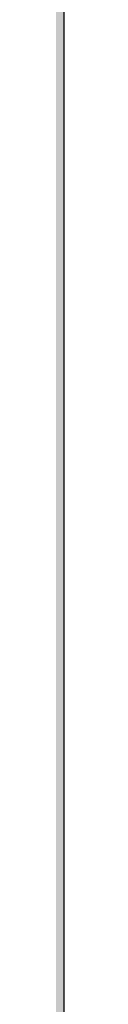
# Model space of a CAD drawing. Units: inches. Extents: x 2091 to 2899, y 967 to 2217.
# Tile 76 of 256: x 2212 to 2212, y 1105 to 1114. Entities that reach past the tile are written whole.
import ezdxf

# ---------------------------------------------------------------- set-up
doc = ezdxf.new("R2010")
doc.units = ezdxf.units.IN
doc.layers.add('A-ANNO-DIMS', color=2, linetype='Continuous', lineweight=18)
doc.layers.add('A-WALL-PATT', color=141, linetype='Continuous', lineweight=13, true_color=0xadddf7)
doc.styles.get("Standard").update_dxf_attribs({"font": 'arial.ttf'})
doc.dimstyles.new('ISO-25', dxfattribs={"dimtxt": 4, "dimasz": 4, "dimexe": 1.25, "dimexo": 0.625, "dimtad": 1, "dimdec": 0, "dimlunit": 3, "dimtxsty": 'Standard', "dimcen": 2.5, "dimadec": 0, "dimazin": 0, "dimtfac": 1, "dimtdec": 0, "dimtmove": 0, "dimatfit": 3, "dimfxl": 1, "dimarcsym": 0})

# ---------------------------------------------------------------- blocks, each defined once
blk = doc.blocks.new('*D71')
at = {"layer": 'A-ANNO-DIMS', "color": 0, "lineweight": -2, "transparency": 16777216}
for p, q in [((2212.1436, 1351.2941), (2212.1436, 969.4643)), ((2452.1436, 1351.2941), (2452.1436, 969.4643)), ((2216.1436, 970.7143), (2448.1436, 970.7143))]:
    blk.add_line(p, q, dxfattribs=at)
at = {"layer": 'A-ANNO-DIMS', "color": 0, "transparency": 16777216}
for points in [[(2216.1436, 971.381), (2216.1436, 970.0476), (2212.1436, 970.7143)], [(2448.1436, 971.381), (2448.1436, 970.0476), (2452.1436, 970.7143)]]:
    blk.add_solid(points, dxfattribs=at)
at = {"layer": 'Defpoints', "color": 0, "transparency": 16777216}
for p in [(2212.1436, 1351.9191), (2452.1436, 1351.9191), (2452.1436, 970.7143)]:
    blk.add_point(p, dxfattribs=at)
at = {"layer": 'A-ANNO-DIMS', "color": 0, "transparency": 16777216, "insert": (2332.1436, 973.3816), "char_height": 4, "attachment_point": 5}
blk.add_mtext('20\'-0"', dxfattribs=at)
blk = doc.blocks.new('*D75')
at = {"layer": 'A-ANNO-DIMS', "color": 0, "lineweight": -2, "transparency": 16777216}
for p, q in [((2212.1436, 1274.7941), (2212.1436, 969.4643)), ((2308.1436, 1274.7941), (2308.1436, 969.4643)), ((2216.1436, 970.7143), (2304.1436, 970.7143))]:
    blk.add_line(p, q, dxfattribs=at)
at = {"layer": 'A-ANNO-DIMS', "color": 0, "transparency": 16777216}
for points in [[(2216.1436, 971.381), (2216.1436, 970.0476), (2212.1436, 970.7143)], [(2304.1436, 971.381), (2304.1436, 970.0476), (2308.1436, 970.7143)]]:
    blk.add_solid(points, dxfattribs=at)
at = {"layer": 'Defpoints', "color": 0, "transparency": 16777216}
for p in [(2212.1436, 1275.4191), (2308.1436, 1275.4191), (2308.1436, 970.7143)]:
    blk.add_point(p, dxfattribs=at)
at = {"layer": 'A-ANNO-DIMS', "color": 0, "transparency": 16777216, "insert": (2260.1436, 973.3816), "char_height": 4, "attachment_point": 5}
blk.add_mtext('8\'-0"', dxfattribs=at)
blk = doc.blocks.new('*D91')
at = {"layer": 'A-ANNO-DIMS', "color": 0, "lineweight": -2, "transparency": 16777216}
for p, q in [((2211.6506, 1152.2471), (2098.3113, 1152.2471)), ((2099.5613, 1103.9191), (2099.5613, 1148.2471)), ((2211.5186, 1099.9191), (2098.3113, 1099.9191))]:
    blk.add_line(p, q, dxfattribs=at)
at = {"layer": 'A-ANNO-DIMS', "color": 0, "transparency": 16777216}
for points in [[(2098.8947, 1148.2471), (2100.228, 1148.2471), (2099.5613, 1152.2471)], [(2098.8947, 1103.9191), (2100.228, 1103.9191), (2099.5613, 1099.9191)]]:
    blk.add_solid(points, dxfattribs=at)
at = {"layer": 'Defpoints', "color": 0, "transparency": 16777216}
for p in [(2099.5613, 1152.2471), (2212.2756, 1152.2471), (2212.1436, 1099.9191)]:
    blk.add_point(p, dxfattribs=at)
at = {"layer": 'A-ANNO-DIMS', "color": 0, "transparency": 16777216, "insert": (2096.8681, 1126.0831), "char_height": 4, "attachment_point": 5, "rotation": 90}
blk.add_mtext('4\'-4 1/2"', dxfattribs=at)

msp = doc.modelspace()

# ---------------------------------------------------------------- hatches: boundary and pattern name
at = {"layer": 'A-WALL-PATT'}
h = msp.add_hatch(color=256, dxfattribs=at)
h.dxf.hatch_style = 1
h.paths.add_polyline_path([(2803.1436, 2050.9191), (2203.1436, 2050.9191), (2203.1436, 1090.9191), (2803.1436, 1090.9191)])
h.paths.add_polyline_path([(2635.7989, 1147.5405), (2674.5241, 1147.5405, 0.376086), (2678.5297, 1152.8802), (2678.5297, 1159.5565, 0.333335), (2674.5243, 1163.5618), (2674.5243, 1163.5619), (2674.5243, 1192.9344), (2635.806, 1192.9344), (2597.0876, 1192.9344), (2597.0876, 1163.5618, 0.333335), (2593.0823, 1159.5565), (2593.0823, 1152.8802, 0.376086), (2597.0879, 1147.5405)], flags=0)
h.paths.add_polyline_path([(2436.0104, 1278.2408, 0.000483), (2435.9526, 1278.215, -0.001328), (2435.9356, 1278.1117, -0.001711), (2436.1164, 1278.0408, 0.002185)], flags=0)
h.paths.add_polyline_path([(2794.1436, 1143.4191), (2794.1436, 1347.4191), (2543.3702, 1347.4191), (2543.3702, 1351.9191), (2794.1436, 1351.9191), (2794.1436, 1392.7136), (2793.9474, 1392.7136), (2793.9474, 1473.5369), (2794.1436, 1473.5369), (2794.1436, 1531.9191), (2650.1436, 1531.9191), (2650.1436, 1536.4191), (2794.1436, 1536.4191), (2794.1436, 1692.4191), (2609.3756, 1692.4191), (2609.3756, 1644.4191), (2604.8756, 1644.4191), (2604.8756, 1744.9191), (2609.3756, 1744.9191), (2609.3756, 1696.9191), (2794.1436, 1696.9191), (2794.1436, 1780.9191), (2609.6436, 1780.9191), (2493.8756, 1780.9191), (2493.8756, 1785.4191), (2609.6436, 1785.4191), (2794.1436, 1785.4191), (2794.1436, 1847.9388), (2793.9512, 1847.9388), (2793.9512, 1928.7622), (2794.1436, 1928.7622), (2794.1436, 1941.4191), (2614.1436, 1941.4191), (2614.1436, 1821.4191), (2609.6436, 1821.4191), (2609.6436, 1941.4191), (2392.1436, 1941.4191), (2392.1436, 1819.9191), (2387.6436, 1819.9191), (2387.6436, 1941.4191), (2212.1436, 1941.4191), (2212.1436, 1783.9191), (2392.1436, 1783.9191), (2392.1436, 1780.9191), (2212.1436, 1780.9191), (2212.1436, 1629.4191), (2387.6436, 1629.4191), (2387.6436, 1744.9191), (2392.1436, 1744.9191), (2392.1436, 1627.9191), (2317.1436, 1627.9191), (2317.1436, 1551.4191), (2317.1436, 1536.4191), (2459.3836, 1536.4191), (2459.3836, 1602.3965), (2463.8836, 1602.3965), (2463.8836, 1531.9191), (2456.6436, 1531.9191), (2456.6436, 1529.9191), (2452.1436, 1529.9191), (2452.1436, 1531.9191), (2312.6436, 1531.9191), (2312.6436, 1551.4191), (2306.1436, 1551.4191), (2306.1436, 1555.9191), (2308.1436, 1555.9191), (2308.1436, 1551.4191), (2312.6436, 1551.4191), (2312.6436, 1627.9191), (2212.1436, 1627.9191), (2212.1436, 1555.9191), (2270.1436, 1555.9191), (2270.1436, 1551.4191), (2212.1436, 1551.4191), (2212.1436, 1351.9191), (2272.1436, 1351.9191), (2272.1436, 1347.4191), (2212.1436, 1347.4191), (2212.1436, 1275.4191), (2308.1436, 1275.4191), (2308.1436, 1351.9191), (2452.1436, 1351.9191), (2452.1436, 1493.9191), (2456.6436, 1493.9191), (2456.6436, 1347.4191), (2312.6436, 1347.4191), (2312.6436, 1270.9191), (2212.1436, 1270.9191), (2212.1436, 1099.9191), (2281.2375, 1099.9191), (2282.871, 1110.9138), (2282.0083, 1116.9966), (2278.5577, 1121.4204), (2268.2056, 1128.0562), (2272.0876, 1128.0562), (2273.8129, 1131.927), (2279.4203, 1134.6919), (2285.0278, 1135.2449), (2287.6158, 1137.4568), (2288.0471, 1138.0098), (2289.3411, 1140.7747), (2291.0665, 1139.6687), (2292.3605, 1135.2449), (2295.3798, 1136.9038), (2296.2425, 1135.7979), (2297.1052, 1133.033), (2300.1246, 1138.0098), (2303.1439, 1138.0098), (2304.4379, 1135.7979), (2303.1439, 1133.586), (2306.5946, 1134.6919), (2307.8887, 1133.033), (2310.908, 1135.2449), (2313.9274, 1134.1389), (2315.6269, 1132.4271), (2308.32, 1117.5496), (2290.2038, 1109.8079), (2288.9098, 1103.1721), (2289.2723, 1099.9191), (2434.9182, 1099.9191), (2431.5932, 1124.7881), (2429.9302, 1169.5531), (2430.9272, 1240.5197), (2435.6589, 1238.1861), (2437.1352, 1196.5541), (2438.7982, 1143.9731), (2442.6782, 1111.9981), (2446.5582, 1099.9191), (2794.1436, 1099.9191), (2794.1436, 1138.9191), (2548.0324, 1138.9191), (2548.0324, 1143.4191), (2548.0324, 1148.8191), (2546.6685, 1148.0316), (2528.6857, 1179.1786, 0.256256), (2512.0324, 1148.8191), (2512.0324, 1143.4191), (2512.0324, 1138.9191), (2507.5324, 1138.9191), (2507.5324, 1143.4191), (2507.5324, 1148.8191, 0.256256), (2490.8792, 1179.1786), (2472.8964, 1148.0316), (2471.5324, 1148.8191), (2471.5324, 1143.4191), (2467.0324, 1143.4191), (2467.0324, 1269.9458, 0.039061), (2460.91, 1273.5801), (2467.0324, 1273.5801), (2467.0324, 1286.3254, 0.014511), (2465.2162, 1286.7619), (2467.0324, 1287.0526), (2467.0324, 1323.4191), (2471.5324, 1323.4191), (2471.5324, 1148.8191), (2489.5324, 1179.996), (2490.8964, 1179.2085), (2490.8792, 1179.1786, -0.256256), (2507.5324, 1148.8191), (2507.5324, 1143.4191), (2512.0324, 1143.4191), (2512.0324, 1148.8191, -0.256256), (2528.6857, 1179.1786), (2528.6685, 1179.2085), (2530.0324, 1179.996), (2548.0324, 1148.8191), (2548.0324, 1143.4191)], flags=16)
h.paths.add_polyline_path([(2607.7685, 1200.9451), (2607.7685, 1265.0306), (2597.0876, 1281.052), (2619.7846, 1281.052), (2627.7953, 1337.1269), (2635.7989, 1337.1269), (2643.8167, 1337.1269), (2651.8274, 1281.052), (2674.5243, 1281.052), (2663.8434, 1265.0306), (2663.8434, 1200.9451), (2635.806, 1200.9451)], flags=0)
edge = h.paths.add_edge_path(flags=0)
edge.add_ellipse((13303.8962, 1272.9987), major_axis=(-10595.313, 0), ratio=0.8423038701, start_angle=0.62823722, end_angle=0.6465541, ccw=False)
edge.add_ellipse((2711.7004, 1156.8527), major_axis=(2.2198, 0), ratio=0.842304, start_angle=111.53524, end_angle=180.62824, ccw=False)
edge.add_ellipse((13303.1563, 1272.9987), major_axis=(-10593.0263, 0), ratio=0.8423038695, start_angle=0.52827147, end_angle=0.6465541, ccw=False)
edge.add_line((2710.7646, 1175.3333), (2710.13, 1175.3333))
edge.add_ellipse((2710.13, 1176.5798), major_axis=(1.4798, 0), ratio=0.842304, start_angle=180, end_angle=270, ccw=False)
edge.add_line((2708.6501, 1176.5798), (2708.6501, 1200.7829))
edge.add_ellipse((2710.13, 1200.7829), major_axis=(1.4798, 0), ratio=0.842304, start_angle=90, end_angle=180, ccw=False)
edge.add_line((2710.13, 1202.0294), (2710.4651, 1202.0294))
edge.add_ellipse((13303.1563, 1272.9987), major_axis=(-10593.0263, 0), ratio=0.8423038695, start_angle=-0.09022909, end_angle=0.38386678, ccw=False)
edge.add_ellipse((2710.13, 1290.927), major_axis=(-1.4798, 0), ratio=0.842304, start_angle=0, end_angle=90, ccw=False)
edge.add_line((2708.6501, 1290.927), (2708.6501, 1315.1302))
edge.add_ellipse((2710.13, 1315.1302), major_axis=(-1.4798, 0), ratio=0.842304, start_angle=-90, end_angle=0, ccw=False)
edge.add_line((2710.13, 1316.3767), (2710.7063, 1316.3767))
edge.add_ellipse((3238.4017, 1296.2896), major_axis=(528.234, 0), ratio=0.84230387, start_angle=176.349572, end_angle=177.82005, ccw=False)
edge.add_ellipse((2775.063, 1071.4507), major_axis=(313.3078, 0), ratio=0.84230387, start_angle=102.125966, end_angle=103.780529, ccw=False)
edge.add_ellipse((2775.063, 1078.3057), major_axis=(-305.3029, 0), ratio=0.84230387, start_angle=-79.790461, end_angle=-77.555373, ccw=False)
edge.add_ellipse((2695.1418, 1541.9754), major_axis=(-250.9602, 0), ratio=0.84230387, start_angle=99.256566, end_angle=102.554933)
edge.add_line((2741.4103, 1334.2143), (2747.1325, 1337.3785))
edge.add_ellipse((2747.5386, 1336.8575), major_axis=(-0.7399, 0), ratio=0.842304, start_angle=270, end_angle=307.93313, ccw=False)
edge.add_ellipse((2747.5386, 1336.8575), major_axis=(-0.7399, 0), ratio=0.842304, start_angle=232.06687, end_angle=270, ccw=False)
edge.add_line((2747.9447, 1337.3785), (2753.6669, 1334.2143))
edge.add_ellipse((2799.9355, 1541.9754), major_axis=(250.9602, 0), ratio=0.84230387, start_angle=257.445067, end_angle=260.743434)
edge.add_ellipse((2720.0142, 1078.3057), major_axis=(305.3029, 0), ratio=0.84230387, start_angle=77.555373, end_angle=79.790461, ccw=False)
edge.add_ellipse((2720.0142, 1071.4507), major_axis=(-313.3078, 0), ratio=0.84230387, start_angle=256.219471, end_angle=257.874034, ccw=False)
edge.add_ellipse((2256.6755, 1296.2896), major_axis=(-528.234, 0), ratio=0.84230387, start_angle=182.17995, end_angle=183.650428, ccw=False)
edge.add_line((2784.3709, 1316.3767), (2784.9472, 1316.3767))
edge.add_ellipse((2784.9472, 1315.1302), major_axis=(1.4798, 0), ratio=0.842304, start_angle=0, end_angle=90, ccw=False)
edge.add_line((2786.4271, 1315.1302), (2786.4271, 1290.927))
edge.add_ellipse((2784.9472, 1290.927), major_axis=(1.4798, 0), ratio=0.842304, start_angle=270, end_angle=360, ccw=False)
edge.add_ellipse((-7808.0791, 1272.9987), major_axis=(10593.0263, 0), ratio=0.8423038695, start_angle=-0.38386678, end_angle=0.09022909, ccw=False)
edge.add_line((2784.6122, 1202.0294), (2784.9472, 1202.0294))
edge.add_ellipse((2784.9472, 1200.7829), major_axis=(1.4798, 0), ratio=0.842304, start_angle=0, end_angle=90, ccw=False)
edge.add_line((2786.4271, 1200.7829), (2786.4271, 1176.5798))
edge.add_ellipse((2784.9472, 1176.5798), major_axis=(-1.4798, 0), ratio=0.842304, start_angle=90, end_angle=180, ccw=False)
edge.add_line((2784.9472, 1175.3333), (2784.3126, 1175.3333))
edge.add_ellipse((-7808.0791, 1272.9987), major_axis=(10593.0263, 0), ratio=0.8423038695, start_angle=-0.6186432, end_angle=-0.52827147, ccw=False)
edge.add_ellipse((2783.3768, 1156.8527), major_axis=(-2.2198, 0), ratio=0.842304, start_angle=179.37176, end_angle=248.46476, ccw=False)
edge.add_ellipse((-7808.819, 1272.9987), major_axis=(-10595.313, 0), ratio=0.8423038658, start_angle=179.35344592, end_angle=179.3717628, ccw=False)
edge.add_ellipse((2780.2973, 1153.5008), major_axis=(-5.2464, 0), ratio=0.842304, start_angle=90, end_angle=179.35345, ccw=False)
edge.add_line((2780.2973, 1149.0817), (2714.7799, 1149.0817))
edge.add_ellipse((2714.7799, 1153.5008), major_axis=(5.2464, 0), ratio=0.842304, start_angle=180.64655, end_angle=270, ccw=False)
edge = h.paths.add_edge_path(flags=0)
edge.add_line((2718.1874, 1151.0078), (2718.1874, 1170.4724))
edge.add_ellipse((2721.1471, 1170.4724), major_axis=(-2.9597, 0), ratio=0.842304, start_angle=-90, end_angle=0, ccw=False)
edge.add_line((2721.1471, 1172.9653), (2773.9302, 1172.9653))
edge.add_ellipse((2773.9302, 1170.4724), major_axis=(-2.9597, 0), ratio=0.842304, start_angle=180, end_angle=270, ccw=False)
edge.add_line((2776.8899, 1170.4724), (2776.8899, 1151.0078))
edge.add_line((2776.8899, 1151.0078), (2718.1874, 1151.0078))
edge = h.paths.add_edge_path(flags=0)
edge.add_line((2718.1874, 1180.2342), (2718.1874, 1199.0578))
edge.add_ellipse((2747.5386, 1320.3986), major_axis=(147.0179, 0), ratio=0.84230387, start_angle=256.401865, end_angle=283.598135)
edge.add_line((2776.8899, 1199.0578), (2776.8899, 1180.2342))
edge.add_ellipse((2747.5386, 1301.575), major_axis=(147.0179, 0), ratio=0.84230387, start_angle=256.401865, end_angle=283.598135, ccw=False)
edge = h.paths.add_edge_path(flags=0)
edge.add_ellipse((13303.1563, 1272.9987), major_axis=(-10591.5465, 0), ratio=0.8423038696, start_angle=0.05559431, end_angle=0.37776419, ccw=False)
edge.add_line((2711.6169, 1262.7217), (2715.6674, 1249.4954))
edge.add_ellipse((6413.892, 1241.6919), major_axis=(-3698.2362, 0), ratio=0.84230387, start_angle=-0.1208974, end_angle=0.3640763)
edge.add_line((2715.761, 1218.1925), (2711.9343, 1203.1674))
edge = h.paths.add_edge_path(flags=0)
edge.add_line((2718.1874, 1251.0746), (2716.0025, 1267.4504))
edge.add_ellipse((2742.1512, 1202.1895), major_axis=(81.7726, 0), ratio=0.8423039, start_angle=94.277421, end_angle=111.834954, ccw=False)
edge.add_line((2737.0097, 1270.9306), (2758.0675, 1270.9306))
edge.add_ellipse((2752.9261, 1202.1895), major_axis=(81.7726, 0), ratio=0.8423039, start_angle=68.165046, end_angle=85.722579, ccw=False)
edge.add_line((2779.0747, 1267.4504), (2776.8899, 1251.0746))
edge.add_ellipse((2750.3381, 1187.8854), major_axis=(79.5797, 0), ratio=0.8423039, start_angle=67.208085, end_angle=85.12993)
edge.add_line((2756.0347, 1254.7437), (2739.0426, 1254.7437))
edge.add_ellipse((2744.7392, 1187.8854), major_axis=(79.5797, 0), ratio=0.8423039, start_angle=94.87007, end_angle=112.791915)
edge = h.paths.add_edge_path(flags=0)
edge.add_line((2783.1429, 1203.1674), (2779.3162, 1218.1925))
edge.add_ellipse((-918.8147, 1241.6919), major_axis=(3698.2362, 0), ratio=0.84230387, start_angle=-0.3640763, end_angle=0.1208974)
edge.add_line((2779.4098, 1249.4954), (2783.4604, 1262.7217))
edge.add_ellipse((-7808.0791, 1272.9987), major_axis=(-10591.5465, 0), ratio=0.8423038695, start_angle=179.62223581, end_angle=179.94440569, ccw=False)
edge = h.paths.add_edge_path(flags=0)
edge.add_ellipse((2734.2009, 1286.6904), major_axis=(-0.3566, 6.3401), ratio=0.603834, start_angle=89.00201, end_angle=253.65741, ccw=False)
edge.add_line((2730.369, 1286.5418), (2730.369, 1301.352))
edge.add_line((2730.369, 1301.352), (2735.9133, 1305.2148))
edge.add_ellipse((2736.3849, 1304.7346), major_axis=(0.7399, 0), ratio=0.842304, start_angle=90, end_angle=134.48021, ccw=False)
edge.add_line((2736.3849, 1305.3578), (2738.0328, 1305.3578))
edge.add_line((2738.0328, 1305.3578), (2738.0328, 1307.7079))
edge.add_ellipse((2794.2016, 1307.7079), major_axis=(56.1689, 0), ratio=0.8423039, start_angle=150.56143, end_angle=180, ccw=False)
edge.add_ellipse((2700.8756, 1307.7079), major_axis=(-56.1689, 0), ratio=0.8423039, start_angle=180, end_angle=209.43857, ccw=False)
edge.add_line((2757.0444, 1307.7079), (2757.0444, 1305.3578))
edge.add_line((2757.0444, 1305.3578), (2758.6923, 1305.3578))
edge.add_ellipse((2758.6923, 1304.7346), major_axis=(-0.7399, 0), ratio=0.842304, start_angle=225.51979, end_angle=270, ccw=False)
edge.add_line((2759.1639, 1305.2148), (2764.7082, 1301.352))
edge.add_line((2764.7082, 1301.352), (2764.7082, 1286.5418))
edge.add_ellipse((2760.8763, 1286.6904), major_axis=(0.3566, 6.3401), ratio=0.603834, start_angle=106.34259, end_angle=270.99799, ccw=False)
edge.add_line((2757.0444, 1285.7971), (2757.0444, 1307.7079))
edge.add_ellipse((2700.8756, 1307.7079), major_axis=(-56.1689, 0), ratio=0.8423039, start_angle=180, end_angle=209.43857)
edge.add_ellipse((2794.2016, 1307.7079), major_axis=(56.1689, 0), ratio=0.8423039, start_angle=150.56143, end_angle=180)
edge.add_line((2738.0328, 1307.7079), (2738.0328, 1285.7971))
h.paths.add_polyline_path([(2417.8123, 1104.4497), (2413.4923, 1102.5297), (2410.6123, 1103.9697), (2409.1723, 1106.3697), (2407.2523, 1107.3297), (2406.2923, 1109.7297), (2405.3323, 1114.0497), (2405.3323, 1117.8897), (2406.2923, 1120.1297), (2407.2523, 1119.8097), (2408.8483, 1118.3277), (2410.1739, 1119.4242), (2410.2113, 1120.4057), (2411.0407, 1121.4191), (2410.6993, 1119.8587), (2410.1739, 1119.4242), (2410.0885, 1117.1761), (2411.1328, 1116.2063), (2413.9723, 1119.3297), (2416.8523, 1120.7697), (2416.8697, 1120.7988), (2417.0351, 1119.4051), (2417.8962, 1118.1434), (2418.2923, 1118.3697), (2419.5444, 1120.0393), (2419.3609, 1118.3875), (2419.0321, 1119.3562), (2418.3989, 1118.5119), (2419.2523, 1114.5297), (2418.7941, 1107.1988)], flags=0)
h.paths.add_polyline_path([(2508.8702, 1347.4191), (2508.3702, 1347.4191), (2508.3702, 1351.9191), (2508.8702, 1351.9191)], flags=0)
h.paths.add_polyline_path([(2473.3702, 1347.4191), (2472.3702, 1347.4191), (2467.8702, 1347.4191), (2467.8702, 1455.4191), (2472.3702, 1455.4191), (2472.3702, 1352.4191), (2473.3702, 1352.4191)], flags=0)
h.paths.add_polyline_path([(2352.1062, 1217.4462), (2349.2262, 1218.8862), (2347.7862, 1221.2862), (2345.8662, 1222.2462), (2344.9062, 1224.6462), (2343.9462, 1228.9662), (2343.9462, 1232.8062), (2344.9062, 1235.0462), (2345.8662, 1234.7262), (2347.4623, 1233.2442), (2348.7879, 1234.3407), (2348.8252, 1235.3222), (2349.6547, 1236.3355), (2349.3132, 1234.7752), (2348.7879, 1234.3407), (2348.7024, 1232.0926), (2349.7468, 1231.1228), (2352.5862, 1234.2462), (2355.4662, 1235.6862), (2355.4837, 1235.7153), (2355.649, 1234.3216), (2356.5102, 1233.0599), (2356.9062, 1233.2862), (2358.1584, 1234.9558), (2357.9749, 1233.304), (2357.6461, 1234.2726), (2357.0129, 1233.4284), (2357.8662, 1229.4462), (2357.4081, 1222.1153), (2356.4262, 1219.3662)], flags=0)
h.paths.add_polyline_path([(2348.2968, 1112.2244), (2347.0138, 1112.3104), (2345.5298, 1114.1274), (2345.7318, 1115.8584), (2346.8118, 1116.9824), (2346.8118, 1114.6464), (2345.8668, 1114.2144), (2346.8798, 1114.3004)], flags=0)
h.paths.add_polyline_path([(2347.0138, 1110.9264), (2346.2718, 1110.4934), (2346.6098, 1111.1864)], flags=0)
h.paths.add_polyline_path([(2345.8668, 1118.1944), (2345.5298, 1117.3294), (2343.7078, 1118.0214), (2344.3828, 1118.6264)], flags=0)
h.paths.add_polyline_path([(2346.6768, 1109.2824), (2346.0698, 1108.0714), (2345.8668, 1110.0614)], flags=0)
h.paths.add_polyline_path([(2345.0568, 1119.7514), (2343.6398, 1119.7514), (2343.9778, 1121.1354)], flags=0)
h.paths.add_polyline_path([(2345.2598, 1116.5504), (2345.1248, 1115.8584), (2344.9218, 1115.6854), (2344.7198, 1116.3774)], flags=0)
h.paths.add_polyline_path([(2345.6648, 1112.3104), (2345.4618, 1111.5324), (2344.0448, 1111.9644), (2344.6518, 1112.5704)], flags=0)
h.paths.add_polyline_path([(2345.1918, 1113.3494), (2344.4498, 1113.8684), (2344.7198, 1114.3874)], flags=0)
h.paths.add_polyline_path([(2344.6518, 1116.8094), (2344.1798, 1115.6854), (2344.6518, 1115.3394), (2343.9098, 1114.9064), (2343.0328, 1115.9444), (2343.6398, 1116.4634)], flags=0)
h.paths.add_polyline_path([(2345.8668, 1106.6864), (2344.9898, 1105.5624), (2344.5168, 1106.6004)], flags=0)
h.paths.add_polyline_path([(2344.8548, 1110.0614), (2344.5168, 1109.2824), (2344.1128, 1109.7154)], flags=0)
h.paths.add_polyline_path([(2344.0448, 1113.5224), (2343.4378, 1113.0894), (2342.7628, 1113.9544)], flags=0)
h.paths.add_polyline_path([(2344.3148, 1111.0124), (2342.9648, 1110.3204), (2342.9648, 1111.0994)], flags=0)
h.paths.add_polyline_path([(2345.1248, 1104.6974), (2344.5848, 1103.7454), (2344.4498, 1104.2644)], flags=0)
h.paths.add_polyline_path([(2342.8298, 1121.2224), (2341.7498, 1120.5304), (2340.5358, 1121.0494), (2340.1308, 1121.8284), (2340.6708, 1122.9524), (2341.1428, 1121.8284), (2341.6148, 1122.0014)], flags=0)
h.paths.add_polyline_path([(2342.9648, 1119.7514), (2343.0328, 1118.4534), (2342.0878, 1118.0214), (2342.0198, 1119.4914)], flags=0)
h.paths.add_polyline_path([(2342.6948, 1116.8964), (2341.9528, 1116.6364), (2342.0198, 1117.3294)], flags=0)
h.paths.add_polyline_path([(2343.0328, 1112.2244), (2342.0198, 1111.7914), (2341.5478, 1112.2244), (2342.3578, 1113.3494)], flags=0)
h.paths.add_polyline_path([(2343.7748, 1104.4374), (2342.6278, 1102.8804), (2342.6948, 1104.6104), (2343.4378, 1105.1294)], flags=0)
h.paths.add_polyline_path([(2342.0198, 1115.0794), (2340.8058, 1115.5124), (2340.9408, 1116.3774)], flags=0)
h.paths.add_polyline_path([(2341.4808, 1120.0974), (2341.4808, 1119.4054), (2341.0758, 1119.5784), (2341.1428, 1120.0974)], flags=0)
h.paths.add_polyline_path([(2341.8178, 1114.4734), (2340.9408, 1113.0894), (2340.8058, 1114.5604)], flags=0)
h.paths.add_polyline_path([(2341.1428, 1118.5404), (2340.9408, 1116.9824), (2339.0508, 1117.6754), (2339.0508, 1118.6264)], flags=0)
h.paths.add_polyline_path([(2342.6948, 1101.6684), (2341.9528, 1101.8414), (2342.5598, 1102.3614)], flags=0)
h.paths.add_polyline_path([(2340.3328, 1119.6654), (2338.4438, 1119.5784), (2337.9038, 1120.3574), (2339.6578, 1120.6164)], flags=0)
h.paths.add_polyline_path([(2340.3328, 1115.3394), (2340.0628, 1113.6954), (2339.3878, 1115.3394)], flags=0)
h.paths.add_polyline_path([(2341.8178, 1103.8314), (2341.5478, 1102.8804), (2341.1428, 1103.6584)], flags=0)
h.paths.add_polyline_path([(2339.0508, 1122.8664), (2337.2958, 1121.8284), (2337.0938, 1123.1254), (2337.7688, 1123.8184)], flags=0)
h.paths.add_polyline_path([(2339.1178, 1121.7414), (2338.8478, 1121.2224), (2338.1738, 1121.0494), (2338.3758, 1121.5684)], flags=0)
h.paths.add_polyline_path([(2339.1858, 1119.3194), (2338.6458, 1118.7134), (2338.2408, 1118.1074), (2338.2408, 1118.8864)], flags=0)
h.paths.add_polyline_path([(2341.1428, 1101.9284), (2340.6028, 1101.2364), (2340.0628, 1101.8414), (2340.6028, 1102.3614)], flags=0)
h.paths.add_polyline_path([(2337.6338, 1117.7614), (2336.6208, 1118.2804), (2337.2958, 1118.9724)], flags=0)
h.paths.add_polyline_path([(2336.8238, 1119.5784), (2334.7988, 1118.9724), (2335.2038, 1120.3574), (2336.5538, 1120.8764)], flags=0)
h.paths.add_polyline_path([(2339.1178, 1100.4574), (2337.3638, 1100.5434), (2336.7558, 1101.2364)], flags=0)
h.paths.add_polyline_path([(2336.3508, 1122.4334), (2336.0138, 1121.9144), (2334.9338, 1122.4334), (2334.5288, 1123.4714), (2335.7438, 1122.7794)], flags=0)
h.paths.add_polyline_path([(2334.7318, 1120.8764), (2334.2588, 1120.3574), (2334.0568, 1120.7894), (2334.5968, 1121.3084)], flags=0)
h.paths.add_polyline_path([(2334.4618, 1122.1744), (2332.5718, 1121.3084), (2331.3568, 1122.1744), (2332.0998, 1122.8664)], flags=0)
h.paths.add_polyline_path([(2334.2588, 1118.5404), (2333.3818, 1118.4534), (2333.6518, 1119.3194)], flags=0)
h.paths.add_polyline_path([(2335.5418, 1102.2744), (2334.1918, 1102.6204), (2335.2718, 1103.3124)], flags=0)
h.paths.add_polyline_path([(2332.7068, 1119.6654), (2331.6948, 1120.4434), (2332.5048, 1120.7894)], flags=0)
h.paths.add_polyline_path([(2334.7318, 1101.1494), (2333.5168, 1101.5824), (2333.9888, 1101.7554)], flags=0)
h.paths.add_polyline_path([(2332.6398, 1116.6364), (2331.0868, 1116.2904), (2331.9648, 1118.1944)], flags=0)
h.paths.add_polyline_path([(2330.7498, 1121.5684), (2330.2768, 1120.2704), (2328.5228, 1119.3194), (2328.9948, 1121.0494)], flags=0)
h.paths.add_polyline_path([(2330.7498, 1118.6264), (2330.0078, 1117.5024), (2329.8728, 1118.0214)], flags=0)
h.paths.add_polyline_path([(2332.0998, 1102.3614), (2330.5468, 1102.0144), (2331.6948, 1102.9664)], flags=0)
h.paths.add_polyline_path([(2329.5348, 1113.6084), (2329.0628, 1112.3104), (2328.5898, 1113.3494)], flags=0)
h.paths.add_polyline_path([(2328.3878, 1117.8484), (2327.5098, 1116.5504), (2327.1728, 1117.7614)], flags=0)
h.paths.add_polyline_path([(2329.7378, 1106.5134), (2329.5348, 1105.3024), (2328.2528, 1106.0814)], flags=0)
h.paths.add_polyline_path([(2328.6578, 1114.3874), (2328.0498, 1114.1274), (2328.3198, 1114.9064)], flags=0)
h.paths.add_polyline_path([(2328.3198, 1112.2244), (2327.1058, 1112.1374), (2326.7008, 1112.6564)], flags=0)
h.paths.add_polyline_path([(2326.9028, 1115.2524), (2326.7008, 1114.1274), (2325.2158, 1113.6084), (2326.0928, 1115.3394)], flags=0)
h.paths.add_polyline_path([(2326.6328, 1108.3304), (2326.0928, 1107.3794), (2325.8908, 1108.5034), (2326.4978, 1109.1094)], flags=0)
h.paths.add_polyline_path([(2615.1436, 1531.9191), (2609.6436, 1531.9191), (2609.6436, 1620.4191), (2614.1436, 1620.4191), (2614.1436, 1536.4191), (2615.1436, 1536.4191)], flags=0)
h.paths.add_polyline_path([(2545.1436, 1563.4191), (2464.1436, 1563.4191), (2464.1436, 1632.4191), (2509.1436, 1632.4191), (2509.1436, 1627.9191), (2509.1436, 1603.9191), (2468.6436, 1603.9191), (2468.6436, 1567.9191), (2540.6436, 1567.9191), (2540.6436, 1591.9191), (2545.1436, 1591.9191)], flags=0)
h.paths.add_polyline_path([(2388.969, 1549.9857), (2357.4342, 1549.9857), (2357.4342, 1623.3608), (2399.3628, 1623.3608), (2435.6895, 1623.3608), (2435.5925, 1602.5593), (2435.5925, 1602.3965), (2388.969, 1602.3965)], flags=0)
h.paths.add_polyline_path([(2388.8806, 1555.8092), (2374.9044, 1555.8092), (2374.9044, 1600.5716), (2374.9044, 1615.4576), (2406.3509, 1615.4576), (2406.3509, 1618.9394), (2412.1743, 1615.4576), (2406.3509, 1611.9759), (2406.3509, 1615.4576), (2388.8806, 1615.4576)], flags=0)
h.paths.add_polyline_path([(2568.8756, 1644.4191), (2453.3756, 1644.4191), (2453.3756, 1785.4191), (2457.8756, 1785.4191), (2457.8756, 1648.9191), (2568.8756, 1648.9191)], flags=0)
h.paths.add_polyline_path([(2212.1436, 1945.9191), (2212.1436, 2041.9191), (2794.1436, 2041.9191), (2794.1436, 1945.9191)], flags=16)
h.paths.add_polyline_path([(2271.0827, 1964.3172), (2776.853, 1964.3172), (2776.853, 2037.1696), (2271.0827, 2037.1696)], flags=8)
h.paths.add_polyline_path([(2380.6493, 1536.8241), (2461.0408, 1536.8241), (2461.0408, 1554.6526), (2380.6493, 1554.6526)], flags=8)
h.paths.add_polyline_path([(2240.7557, 1609.7255), (2309.1858, 1609.7255), (2309.1858, 1617.6982), (2240.7557, 1617.6982)], flags=8)
h.paths.add_polyline_path([(2212.6773, 1313.5041), (2282.5915, 1313.5041), (2282.5915, 1322.7452), (2212.6773, 1322.7452)], flags=8)
h.paths.add_polyline_path([(2457.112, 1114.7786), (2558.4816, 1114.7786), (2558.4816, 1142.2197), (2457.112, 1142.2197)], flags=8)
h.paths.add_polyline_path([(2473.4423, 1273.0101), (2604.6412, 1273.0101), (2604.6412, 1318.3469), (2473.4423, 1318.3469)], flags=8)
h.paths.add_polyline_path([(2638.8763, 1626.9774), (2684.2504, 1627.9767), (2684.0385, 1637.5975), (2638.6644, 1636.5982)], flags=8)
h.paths.add_polyline_path([(2537.5906, 1453.7934), (2628.3895, 1453.7934), (2628.3895, 1475.3448), (2537.5906, 1475.3448)], flags=8)
h.paths.add_polyline_path([(2504.1376, 1714.6324), (2554.6472, 1714.6324), (2554.6472, 1730.2377), (2504.1376, 1730.2377)], flags=8)
h.paths.add_polyline_path([(2487.5012, 1575.6519), (2535.0971, 1575.6519), (2535.0971, 1598.3776), (2487.5012, 1598.3776)], flags=8)
h.paths.add_polyline_path([(2709.0994, 1735.7103), (2740.0166, 1735.7103), (2740.0166, 1749.9376), (2709.0994, 1749.9376)], flags=8)
h.paths.add_polyline_path([(2442.4384, 1792.1717), (2564.7288, 1792.1717), (2564.7288, 1842.0002), (2442.4384, 1842.0002)], flags=8)
h.paths.add_polyline_path([(2655.8158, 1809.6441), (2789.5201, 1806.6938), (2790.085, 1832.2916), (2656.3806, 1835.2419)], flags=8)
h.paths.add_polyline_path([(2234.8427, 1797.7201), (2368.5929, 1794.7689), (2369.1607, 1820.5041), (2235.4106, 1823.4554)], flags=8)
h.paths.add_polyline_path([(2245.1385, 1644.0063), (2398.4277, 1640.6239), (2398.9948, 1666.3248), (2245.7056, 1669.7073)], flags=8)
h.paths.add_polyline_path([(2306.1428, 1431.1685), (2413.7683, 1428.7937), (2414.3331, 1454.3915), (2306.7077, 1456.7664)], flags=8)
h.paths.add_polyline_path([(2306.8346, 1458.2331), (2393.3805, 1456.3234), (2393.9328, 1481.3544), (2307.3869, 1483.2641)], flags=8)

# ---------------------------------------------------------------- dimensions: what is measured, and where the dimension line sits
at = {"layer": 'A-ANNO-DIMS'}
for base, p1, p2, picture, middle in [((2452.1436, 970.7143), (2212.1436, 1351.9191), (2452.1436, 1351.9191), '*D71', (2332.1436, 973.3816)), ((2308.1436, 970.7143), (2212.1436, 1275.4191), (2308.1436, 1275.4191), '*D75', (2260.1436, 973.3816))]:
    dim = msp.add_linear_dim(base=base, p1=p1, p2=p2, dimstyle='ISO-25', override={"dimdec": 1, "dimlfac": 1, "dimrnd": 0, "dimzin": 1, "dimdsep": 46, "dimlunit": 4, "dimfrac": 2}, dxfattribs=at)
    dim.commit()
    dim.dimension.update_dxf_attribs({"geometry": picture, "text_midpoint": middle})
dim = msp.add_linear_dim(base=(2099.5613, 1152.2471), p1=(2212.1436, 1099.9191), p2=(2212.2756, 1152.2471), angle=90, dimstyle='ISO-25', override={"dimdec": 1, "dimlfac": 1, "dimrnd": 0, "dimzin": 1, "dimdsep": 46, "dimlunit": 4, "dimfrac": 2}, dxfattribs=at)
dim.commit()
dim.dimension.update_dxf_attribs({"geometry": '*D91', "text_midpoint": (2096.8681, 1126.0831)})

doc.saveas('drawing.dxf')
